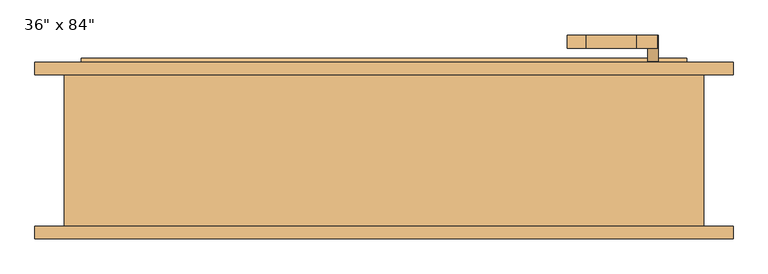
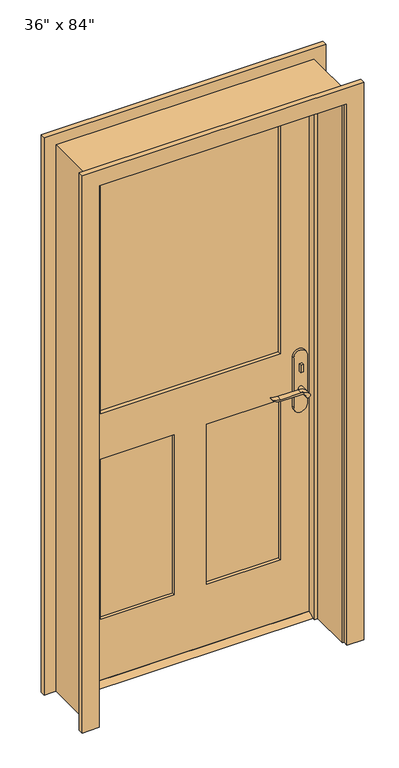
"""IFC4 building model written with IfcOpenShell, lengths in millimetres: door geometry."""

from ifc_helpers import new_model, si_unit, point, frame, frame_2d, origin, place, context, project, spatial, polyline, circle_curve, trimmed, segment, composite_curve, outline, extrude, faceted_brep, source, transform, mapped, element, save


def door_b46a707d(model_context):
    return source(origin(), model_context, "Body", "SolidModel", [
        extrude(outline(polyline([(76.2, 12.7), (111.125, 12.7), (136.525, 0.0), (50.8, 0.0), (76.2, 12.7)])), frame((-457.2, 0.0, 0.0), z_axis=(1.0, 0.0, 0.0), x_axis=(0.0, 1.0, 0.0)), (0.0, 0.0, 1.0), 914.4),
        extrude(outline(polyline([(411.4, 56.2), (401.4, 56.2), (401.4, 66.2), (411.4, 66.2), (411.4, 56.2)])), frame((0.0, 0.0, 981.9), z_axis=(0.0, 0.0, 1.0), x_axis=(1.0, 0.0, 0.0)), (0.0, 0.0, 1.0), 30.0),
        extrude(outline(composite_curve([segment(trimmed(circle_curve(frame_2d((996.9, 406.4)), 8.0), [point((996.9, 398.4))], [point((996.9, 414.4))], False, "CARTESIAN"), True, "CONTINUOUS"), segment(trimmed(circle_curve(frame_2d((996.9, 406.4)), 8.0), [point((996.9, 414.4))], [point((996.9, 398.4))], False, "CARTESIAN"), True, "CONTINUOUS")], self_intersect=False)), frame((0.0, 121.125, 0.0), z_axis=(0.0, 1.0, 0.0), x_axis=(0.0, 0.0, 1.0)), (0.0, 0.0, 1.0), 10.0),
        extrude(outline(composite_curve([segment(trimmed(circle_curve(frame_2d((897.1555521, 382.7324871)), 37.2832219), [point((919.0523287, 412.9081363))], [point((934.4, 381.0325667))], False, "CARTESIAN"), True, "CONTINUOUS"), segment(polyline([(934.4, 381.0325667), (934.4, 304.7564091)]), True, "CONTINUOUS"), segment(trimmed(circle_curve(frame_2d((1017.6850638, 304.8227909)), 83.2850902), [point((934.4, 304.7564091))], [point((939.4, 276.4))], True, "CARTESIAN"), True, "CONTINUOUS"), segment(polyline([(939.4, 276.4), (936.6135558, 276.4)]), True, "CONTINUOUS"), segment(trimmed(circle_curve(frame_2d((986.6709207, 308.3396612)), 59.3791355), [point((936.6135558, 276.4))], [point((927.4, 304.7564091))], False, "CARTESIAN"), True, "CONTINUOUS"), segment(polyline([(927.4, 304.7564091), (927.4, 381.0138099)]), True, "CONTINUOUS"), segment(trimmed(circle_curve(frame_2d((909.2738613, 381.0138099)), 18.1261387), [point((927.4, 381.0138099))], [point((914.4, 398.4))], True, "CARTESIAN"), True, "CONTINUOUS"), segment(trimmed(circle_curve(frame_2d((914.4, 406.4)), 8.0), [point((914.4, 398.4))], [point((919.0523287, 412.9081363))], False, "CARTESIAN"), True, "CONTINUOUS")], self_intersect=False)), frame((0.0, 16.2, 0.0), z_axis=(0.0, 1.0, 0.0), x_axis=(0.0, 0.0, 1.0)), (0.0, 0.0, 1.0), 20.0),
        extrude(outline(composite_curve([segment(trimmed(circle_curve(frame_2d((914.4, 406.4)), 8.0), [point((914.3999903, 398.4))], [point((919.0523287, 412.9081363))], False, "CARTESIAN"), True, "CONTINUOUS"), segment(trimmed(circle_curve(frame_2d((897.1555521, 382.7324871)), 37.2832219), [point((919.0523287, 412.9081363))], [point((934.4, 381.0325667))], False, "CARTESIAN"), True, "CONTINUOUS"), segment(polyline([(934.4, 381.0325667), (934.4, 304.7564091)]), True, "CONTINUOUS"), segment(trimmed(circle_curve(frame_2d((1017.6850638, 304.8227909)), 83.2850902), [point((934.4, 304.7564091))], [point((939.4, 276.4))], True, "CARTESIAN"), True, "CONTINUOUS"), segment(polyline([(939.4, 276.4), (936.6135558, 276.4)]), True, "CONTINUOUS"), segment(trimmed(circle_curve(frame_2d((986.6709207, 308.3396612)), 59.3791355), [point((936.6135558, 276.4))], [point((927.4, 304.7564091))], False, "CARTESIAN"), True, "CONTINUOUS"), segment(polyline([(927.4, 304.7564091), (927.4, 381.0138122)]), True, "CONTINUOUS"), segment(trimmed(circle_curve(frame_2d((909.2738682, 381.0138122)), 18.1261318), [point((927.4, 381.0138122))], [point((914.3999903, 398.4))], True, "CARTESIAN"), True, "CONTINUOUS")], self_intersect=False)), frame((0.0, 151.125, 0.0), z_axis=(0.0, 1.0, 0.0), x_axis=(0.0, 0.0, 1.0)), (0.0, 0.0, 1.0), 20.0),
        extrude(outline(composite_curve([segment(trimmed(circle_curve(frame_2d((914.4, 406.4)), 8.0), [point((914.4, 398.4))], [point((914.4, 414.4))], False, "CARTESIAN"), True, "CONTINUOUS"), segment(trimmed(circle_curve(frame_2d((914.4, 406.4)), 8.0), [point((914.4, 414.4))], [point((914.4, 398.4))], False, "CARTESIAN"), True, "CONTINUOUS")], self_intersect=False)), frame((0.0, 36.2, 0.0), z_axis=(0.0, 1.0, 0.0), x_axis=(0.0, 0.0, 1.0)), (0.0, 0.0, 1.0), 30.0),
        extrude(outline(composite_curve([segment(trimmed(circle_curve(frame_2d((914.4, 406.4)), 8.0), [point((914.4, 398.4))], [point((914.4, 414.4))], False, "CARTESIAN"), True, "CONTINUOUS"), segment(trimmed(circle_curve(frame_2d((914.4, 406.4)), 8.0), [point((914.4, 414.4))], [point((914.4, 398.4))], False, "CARTESIAN"), True, "CONTINUOUS")], self_intersect=False)), frame((0.0, 121.125, 0.0), z_axis=(0.0, 1.0, 0.0), x_axis=(0.0, 0.0, 1.0)), (0.0, 0.0, 1.0), 30.0),
        extrude(outline(composite_curve([segment(polyline([(844.4, 431.4), (1039.4, 431.4)]), True, "CONTINUOUS"), segment(trimmed(circle_curve(frame_2d((1039.4, 406.4)), 25.0), [point((1039.4, 431.4))], [point((1039.4, 381.4))], False, "CARTESIAN"), True, "CONTINUOUS"), segment(polyline([(1039.4, 381.4), (844.4, 381.4)]), True, "CONTINUOUS"), segment(trimmed(circle_curve(frame_2d((844.4, 406.4)), 25.0), [point((844.4, 381.4))], [point((844.4, 431.4))], False, "CARTESIAN"), True, "CONTINUOUS")], self_intersect=False)), frame((0.0, 66.2, 0.0), z_axis=(0.0, 1.0, 0.0), x_axis=(0.0, 0.0, 1.0)), (0.0, 0.0, 1.0), 10.0),
        extrude(outline(composite_curve([segment(polyline([(844.4, 431.4), (1039.4, 431.4)]), True, "CONTINUOUS"), segment(trimmed(circle_curve(frame_2d((1039.4, 406.4)), 25.0), [point((1039.4, 431.4))], [point((1039.4, 381.4))], False, "CARTESIAN"), True, "CONTINUOUS"), segment(polyline([(1039.4, 381.4), (844.4, 381.4)]), True, "CONTINUOUS"), segment(trimmed(circle_curve(frame_2d((844.4, 406.4)), 25.0), [point((844.4, 381.4))], [point((844.4, 431.4))], False, "CARTESIAN"), True, "CONTINUOUS")], self_intersect=False)), frame((0.0, 111.125, 0.0), z_axis=(0.0, 1.0, 0.0), x_axis=(0.0, 0.0, 1.0)), (0.0, 0.0, 1.0), 10.0),
        extrude(outline(polyline([(2133.6, -457.2), (12.7, -457.2), (12.7, 457.2), (2133.6, 457.2), (2133.6, -457.2)]), holes=[polyline([(1066.8, -336.55), (2012.95, -336.55), (2012.95, 336.55), (1066.8, 336.55), (1066.8, -336.55)]), polyline([(885.825, -60.325), (254.0, -60.325), (254.0, -336.55), (885.825, -336.55), (885.825, -60.325)]), polyline([(885.825, 336.55), (254.0, 336.55), (254.0, 60.325), (885.825, 60.325), (885.825, 336.55)])]), frame((0.0, 76.2, 0.0), z_axis=(0.0, 1.0, 0.0), x_axis=(0.0, 0.0, 1.0)), (0.0, 0.0, 1.0), 34.925),
        faceted_brep([(482.6, 111.125, 0.0), (482.6, -117.475, 0.0), (457.2, -117.475, 0.0), (457.2, 41.275, 0.0), (444.5, 41.275, 0.0), (444.5, 76.2, 0.0), (457.2, 76.2, 0.0), (457.2, 111.125, 0.0), (482.6, 111.125, 2159.0), (482.6, -117.475, 2159.0), (-482.6, -117.475, 2159.0), (-482.6, -117.475, 0.0), (-457.2, -117.475, 0.0), (-457.2, -117.475, 2133.6), (457.2, -117.475, 2133.6), (457.2, 41.275, 2133.6), (-457.2, 41.275, 2133.6), (-457.2, 41.275, 0.0), (-444.5, 41.275, 0.0), (-444.5, 41.275, 2120.9), (444.5, 41.275, 2120.9), (444.5, 76.2, 2120.9), (-444.5, 76.2, 2120.9), (-444.5, 76.2, 0.0), (-457.2, 76.2, 0.0), (-457.2, 76.2, 2133.6), (457.2, 76.2, 2133.6), (457.2, 111.125, 2133.6), (-457.2, 111.125, 2133.6), (-457.2, 111.125, 0.0), (-482.6, 111.125, 0.0), (-482.6, 111.125, 2159.0)], [[[0, 1, 2, 3, 4, 5, 6, 7]], [[1, 0, 8, 9]], [[2, 1, 9, 10, 11, 12, 13, 14]], [[3, 2, 14, 15]], [[4, 3, 15, 16, 17, 18, 19, 20]], [[5, 4, 20, 21]], [[6, 5, 21, 22, 23, 24, 25, 26]], [[7, 6, 26, 27]], [[0, 7, 27, 28, 29, 30, 31, 8]], [[9, 8, 31, 10]], [[15, 14, 13, 16]], [[21, 20, 19, 22]], [[27, 26, 25, 28]], [[30, 29, 24, 23, 18, 17, 12, 11]], [[10, 31, 30, 11]], [[16, 13, 12, 17]], [[22, 19, 18, 23]], [[28, 25, 24, 29]]]),
        extrude(outline(polyline([(-60.325, 87.8416667), (-336.55, 87.8416667), (-336.55, 99.4833333), (-60.325, 99.4833333), (-60.325, 87.8416667)])), frame((0.0, 0.0, 254.0), z_axis=(0.0, 0.0, 1.0), x_axis=(1.0, 0.0, 0.0)), (0.0, 0.0, 1.0), 631.825),
        extrude(outline(polyline([(336.55, 87.8416667), (60.325, 87.8416667), (60.325, 99.4833333), (336.55, 99.4833333), (336.55, 87.8416667)])), frame((0.0, 0.0, 254.0), z_axis=(0.0, 0.0, 1.0), x_axis=(1.0, 0.0, 0.0)), (0.0, 0.0, 1.0), 631.825),
        extrude(outline(polyline([(336.55, 90.17), (-336.55, 90.17), (-336.55, 97.155), (336.55, 97.155), (336.55, 90.17)])), frame((0.0, 0.0, 1066.8), z_axis=(0.0, 0.0, 1.0), x_axis=(1.0, 0.0, 0.0)), (0.0, 0.0, 1.0), 946.15),
        extrude(outline(polyline([(0.0, -527.05), (0.0, -463.55), (2139.95, -463.55), (2139.95, 463.55), (0.0, 463.55), (0.0, 527.05), (2203.45, 527.05), (2203.45, -527.05), (0.0, -527.05)])), frame((0.0, -136.525, 0.0), z_axis=(0.0, 1.0, 0.0), x_axis=(0.0, 0.0, 1.0)), (0.0, 0.0, 1.0), 19.05),
        extrude(outline(polyline([(0.0, -527.05), (0.0, -463.55), (2139.95, -463.55), (2139.95, 463.55), (0.0, 463.55), (0.0, 527.05), (2203.45, 527.05), (2203.45, -527.05), (0.0, -527.05)])), frame((0.0, 111.125, 0.0), z_axis=(0.0, 1.0, 0.0), x_axis=(0.0, 0.0, 1.0)), (0.0, 0.0, 1.0), 19.05),
    ])


if __name__ == "__main__":
    model = new_model("IFC4")
    model_context = context("Model", 3, world=origin())
    ifc_project = project(units=[si_unit("LENGTHUNIT", "METRE", prefix="MILLI")], contexts=[model_context])
    site = spatial("IfcSite", under=ifc_project)
    building = spatial("IfcBuilding", under=site)
    placement = place(None, origin())
    door_shape = door_b46a707d(model_context)
    element("IfcDoor", 1, ObjectType="36\" x 84\"", at=placement, inside=building, context=model_context, shape_type="MappedRepresentation", body=[
        mapped(door_shape, transform((0.0, 0.0, 0.0), x_axis=(1.0, 0.0, 0.0), y_axis=(0.0, 1.0, 0.0), z_axis=(0.0, 0.0, 1.0))),
    ])
    save(model, "model.ifc")

# Revit data of these elements
# Type "36\" x 84\""
#   Type Mark = "9"
#   Assembly Code = "B2030100"
#   Analytic Construction = "French door, wood frame with single glass"
#   Top Rail = 0' - 4 3/4"
#   Threshold Offset [instance default] = 0' - 0 1/2"
#   Thickness = 0' - 1 3/8"
#   Thermal Resistance (R) = 1.0696 (h·ft²·°F)/BTU
#   Swing Angle [instance default] = 90.00°
#   Stiles = 0' - 4 3/4"
#   Rough Width = 3' - 2"
#   Rough Height = 7' - 1"
#   Lock Rail = 0' - 7 1/8"
#   Height = 7' - 0"
#   Width = 3' - 0"
#   Heat Transfer Coefficient (U) = 0.9350 BTU/(h·ft²·°F)
#   Door Offset [instance default] = 0' - 0"
#   Bottom Rail = 0' - 9 1/2"
#   Threshold [instance default] = yes
#   Function = 1
#   Exterior Trim [instance default] = yes
#   Trim Material = Cherry
#   Threshold Material = Cherry
#   Panel Material = Cherry
#   Glazing = Glass
#   Frame Material = Cherry
#   Door Handle Material = Aluminum
#   Visual Light Transmittance = 0
#   Solar Heat Gain Coefficient = 0
#   Wall Closure = (empty or 0)
#   Construction Type = (empty or 0)
# Element 1 (IfcDoor, "36\" x 84\"")
#   Materials on its faces: "Cherry", "Aluminum", "Glass"
# Materials
#   "Cherry": class "Wood", colour RGB 226 177 128, transparency 0, Description = "Prunus Serotina", Cost = 0
#   "Glass": class "Glass", colour RGB 0 128 192, transparency 0.75, Description = "Soda Lime Glass", Cost = 0
#   "Aluminum": class "Metal", colour RGB 247 247 247, transparency 0, Description = "Aluminum 6061", Cost = 0
